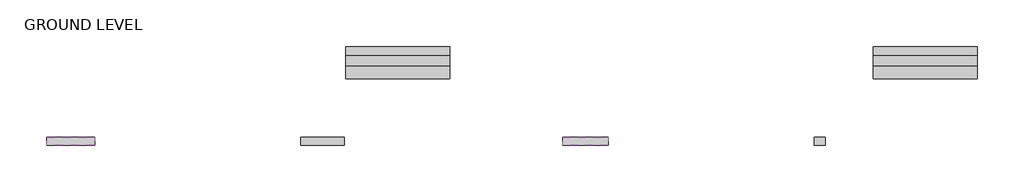
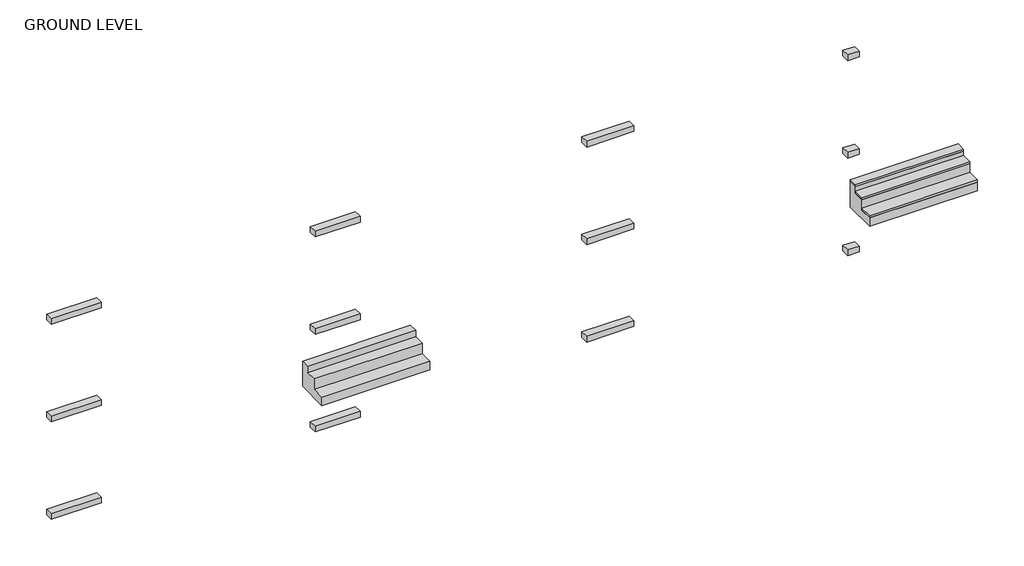
# One storey: 9 proxies.
"""IFC4 building model written with IfcOpenShell, lengths in millimetres."""

from ifc_helpers import new_model, si_unit, frame, origin, place, context, project, spatial, polyline, outline, extrude, transform, mapped, element, save
from components import generic_models_5_generic_models_5_28bce95b

model = new_model("IFC4")

# Units and contexts
model_context = context("Model", 3, world=origin())
ifc_project = project(units=[si_unit("LENGTHUNIT", "METRE", prefix="MILLI")], contexts=[model_context])

# Site, building, storey
site = spatial("IfcSite", under=ifc_project)
building = spatial("IfcBuilding", under=site)
storey = spatial("IfcBuildingStorey", under=building, Name="GROUND LEVEL", Elevation=0.0)

# Proxies
placement = place(None, origin())
generic_models_5_generic_models_5_shape = generic_models_5_generic_models_5_28bce95b(model_context)
element("IfcBuildingElementProxy", 1, Name="Generic Models 5 : Generic Models 5", ObjectType="Generic Models 5 : Generic Models 5", at=placement, inside=storey, context=model_context, shape_type="MappedRepresentation", body=[
    mapped(generic_models_5_generic_models_5_shape, transform((0.0, 0.0, 0.0), x_axis=(1.0, 0.0, 0.0), y_axis=(0.0, 1.0, 0.0), z_axis=(0.0, 0.0, 1.0))),
])
element("IfcBuildingElementProxy", 2, Name="Generic Models 6 : Generic Models 5", ObjectType="Generic Models 6 : Generic Models 5", at=placement, inside=storey, context=model_context, shape_type="MappedRepresentation", body=[
    mapped(generic_models_5_generic_models_5_shape, transform((0.0, 0.0, 25.4), x_axis=(1.0, 0.0, 0.0), y_axis=(0.0, 1.0, 0.0), z_axis=(0.0, 0.0, 1.0))),
])
element("IfcBuildingElementProxy", 3, Name="Generic Models 7 : Generic Models 5", ObjectType="Generic Models 7 : Generic Models 5", at=placement, inside=storey, context=model_context, shape_type="MappedRepresentation", body=[
    mapped(generic_models_5_generic_models_5_shape, transform((-6248.4, 0.0, 25.4), x_axis=(1.0, 0.0, 0.0), y_axis=(0.0, 1.0, 0.0), z_axis=(0.0, 0.0, 1.0))),
])
element("IfcBuildingElementProxy", 4, Name="Reveal 2", ObjectType="Reveal 2", at=placement, inside=storey, context=model_context, shape_type="SweptSolid", body=[
    extrude(outline(polyline([(-15253.3007021, -5496.2840801), (-15253.3007021, -5404.2090801), (-14738.9507021, -5404.2090801), (-14738.9507021, -5496.2840801), (-15253.3007021, -5496.2840801)])), frame((0.0, 0.0, 368.3), z_axis=(0.0, 0.0, 1.0), x_axis=(1.0, 0.0, 0.0)), (0.0, 0.0, 1.0), 67.7333333),
    extrude(outline(polyline([(-18263.2007021, -5496.2840801), (-18263.2007021, -5404.2090801), (-17691.7007021, -5404.2090801), (-17691.7007021, -5496.2840801), (-18263.2007021, -5496.2840801)])), frame((0.0, 0.0, 368.3), z_axis=(0.0, 0.0, 1.0), x_axis=(1.0, 0.0, 0.0)), (0.0, 0.0, 1.0), 67.7333333),
])
element("IfcBuildingElementProxy", 5, Name="Reveal 2", ObjectType="Reveal 2", at=placement, inside=storey, context=model_context, shape_type="SweptSolid", body=[
    extrude(outline(polyline([(-15253.3007021, -5496.2840801), (-15253.3007021, -5404.2090801), (-14738.9507021, -5404.2090801), (-14738.9507021, -5496.2840801), (-15253.3007021, -5496.2840801)])), frame((0.0, 0.0, 2720.34), z_axis=(0.0, 0.0, 1.0), x_axis=(1.0, 0.0, 0.0)), (0.0, 0.0, 1.0), 67.7333333),
    extrude(outline(polyline([(-18263.2007021, -5496.2840801), (-18263.2007021, -5404.2090801), (-17691.7007021, -5404.2090801), (-17691.7007021, -5496.2840801), (-18263.2007021, -5496.2840801)])), frame((0.0, 0.0, 2720.34), z_axis=(0.0, 0.0, 1.0), x_axis=(1.0, 0.0, 0.0)), (0.0, 0.0, 1.0), 67.7333333),
])
element("IfcBuildingElementProxy", 6, Name="Reveal 2", ObjectType="Reveal 2", at=placement, inside=storey, context=model_context, shape_type="SweptSolid", body=[
    extrude(outline(polyline([(-15253.3007021, -5496.2840801), (-15253.3007021, -5404.2090801), (-14738.9507021, -5404.2090801), (-14738.9507021, -5496.2840801), (-15253.3007021, -5496.2840801)])), frame((0.0, 0.0, 1544.32), z_axis=(0.0, 0.0, 1.0), x_axis=(1.0, 0.0, 0.0)), (0.0, 0.0, 1.0), 67.7333333),
    extrude(outline(polyline([(-18263.2007021, -5496.2840801), (-18263.2007021, -5404.2090801), (-17691.7007021, -5404.2090801), (-17691.7007021, -5496.2840801), (-18263.2007021, -5496.2840801)])), frame((0.0, 0.0, 1544.32), z_axis=(0.0, 0.0, 1.0), x_axis=(1.0, 0.0, 0.0)), (0.0, 0.0, 1.0), 67.7333333),
])
element("IfcBuildingElementProxy", 7, Name="Reveal 2", ObjectType="Reveal 2", at=placement, inside=storey, context=model_context, shape_type="SweptSolid", body=[
    extrude(outline(polyline([(-9044.8860997, -5404.2090801), (-9044.8860997, -5496.2840801), (-9176.5344894, -5496.2840801), (-9176.5344894, -5404.2090801), (-9044.8860997, -5404.2090801)])), frame((0.0, 0.0, 368.3), z_axis=(0.0, 0.0, 1.0), x_axis=(1.0, 0.0, 0.0)), (0.0, 0.0, 1.0), 67.7333333),
    extrude(outline(polyline([(-11614.9344894, -5404.2090801), (-11614.9344894, -5496.2840801), (-12154.5007021, -5496.2840801), (-12154.5007021, -5404.2090801), (-11614.9344894, -5404.2090801)])), frame((0.0, 0.0, 368.3), z_axis=(0.0, 0.0, 1.0), x_axis=(1.0, 0.0, 0.0)), (0.0, 0.0, 1.0), 67.7333333),
])
element("IfcBuildingElementProxy", 8, Name="Reveal 2", ObjectType="Reveal 2", at=placement, inside=storey, context=model_context, shape_type="SweptSolid", body=[
    extrude(outline(polyline([(-9044.8860997, -5404.2090801), (-9044.8860997, -5496.2840801), (-9176.5344894, -5496.2840801), (-9176.5344894, -5404.2090801), (-9044.8860997, -5404.2090801)])), frame((0.0, 0.0, 2720.34), z_axis=(0.0, 0.0, 1.0), x_axis=(1.0, 0.0, 0.0)), (0.0, 0.0, 1.0), 67.7333333),
    extrude(outline(polyline([(-11614.9344894, -5404.2090801), (-11614.9344894, -5496.2840801), (-12154.5007021, -5496.2840801), (-12154.5007021, -5404.2090801), (-11614.9344894, -5404.2090801)])), frame((0.0, 0.0, 2720.34), z_axis=(0.0, 0.0, 1.0), x_axis=(1.0, 0.0, 0.0)), (0.0, 0.0, 1.0), 67.7333333),
])
element("IfcBuildingElementProxy", 9, Name="Reveal 2", ObjectType="Reveal 2", at=placement, inside=storey, context=model_context, shape_type="SweptSolid", body=[
    extrude(outline(polyline([(-9044.8860997, -5404.2090801), (-9044.8860997, -5496.2840801), (-9176.5344894, -5496.2840801), (-9176.5344894, -5404.2090801), (-9044.8860997, -5404.2090801)])), frame((0.0, 0.0, 1544.32), z_axis=(0.0, 0.0, 1.0), x_axis=(1.0, 0.0, 0.0)), (0.0, 0.0, 1.0), 67.7333333),
    extrude(outline(polyline([(-11614.9344894, -5404.2090801), (-11614.9344894, -5496.2840801), (-12154.5007021, -5496.2840801), (-12154.5007021, -5404.2090801), (-11614.9344894, -5404.2090801)])), frame((0.0, 0.0, 1544.32), z_axis=(0.0, 0.0, 1.0), x_axis=(1.0, 0.0, 0.0)), (0.0, 0.0, 1.0), 67.7333333),
])

save(model, "model.ifc")

# Revit data of these elements
# Element 1 (IfcBuildingElementProxy, "Generic Models 5 : Generic Models 5")
#   Phase Created = New Construction
# Element 2 (IfcBuildingElementProxy, "Generic Models 6 : Generic Models 5")
#   Phase Created = New Construction
# Element 3 (IfcBuildingElementProxy, "Generic Models 7 : Generic Models 5")
#   Phase Created = New Construction
